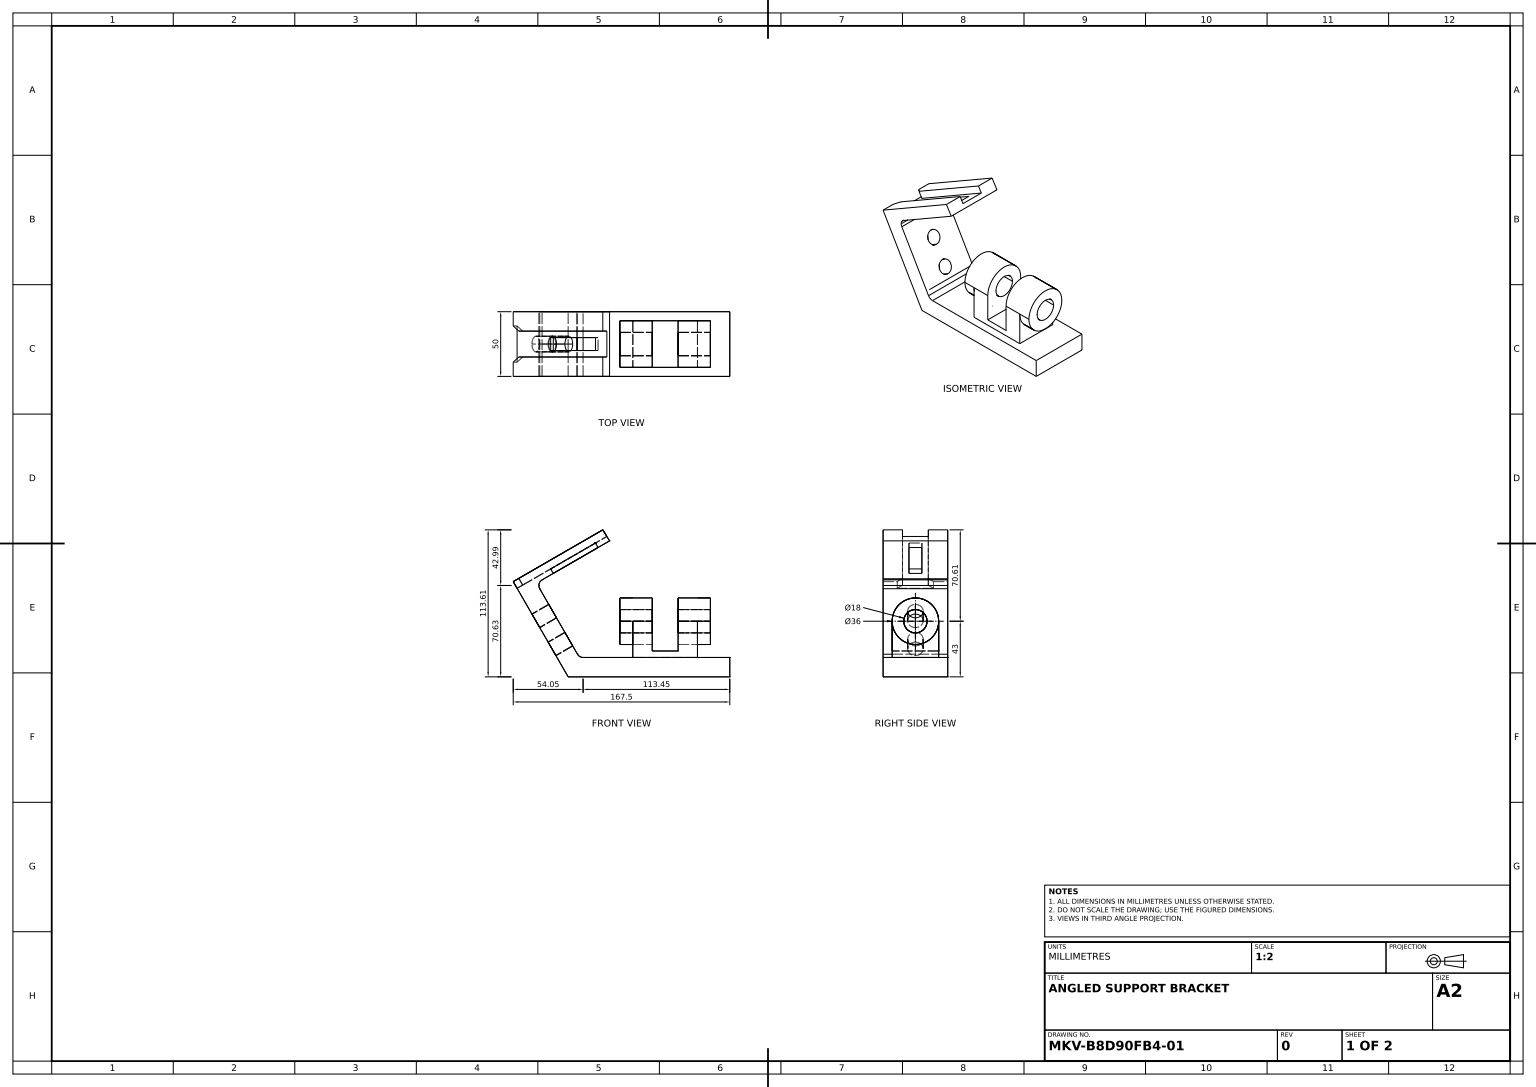
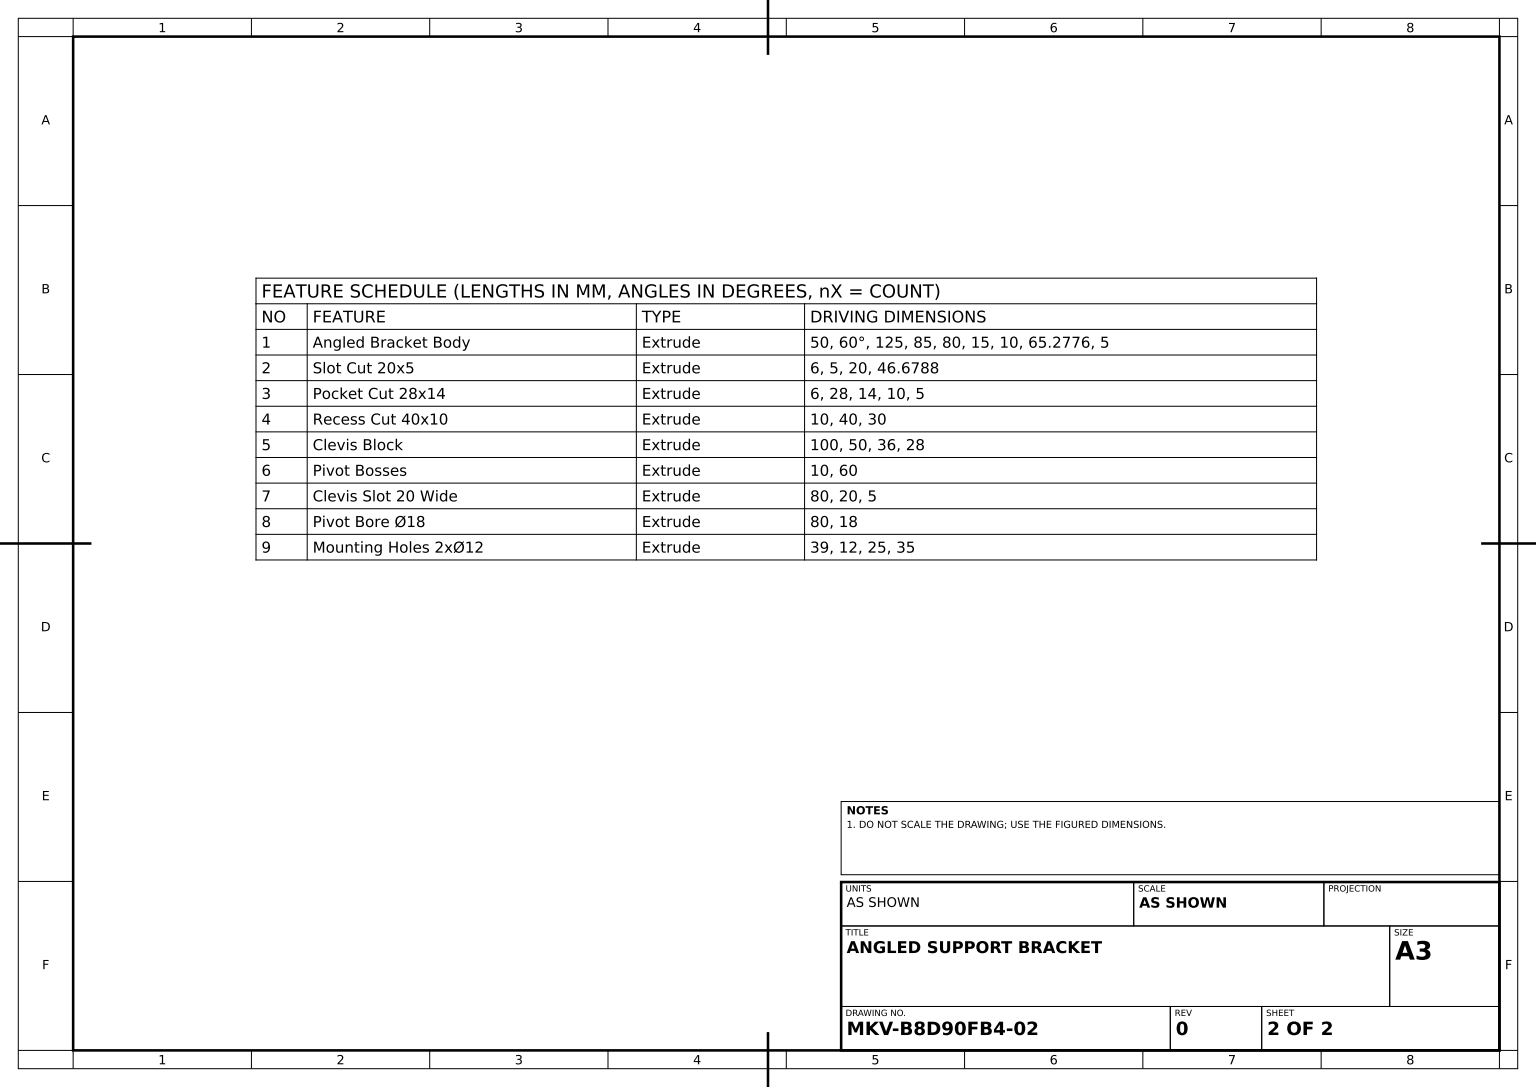
SolidWorks part; units mm, degrees
material "Plain Carbon Steel"
ref_plane "Front Plane" through (0, 0, 0) normal (0, 0, 1) x (1, 0, 0)
ref_plane "Top Plane" through (0, 0, 0) normal (0, 1, 0) x (1, 0, 0)
ref_plane "Right Plane" through (0, 0, 0) normal (1, 0, 0) x (0, 0, -1)
sketch "Bracket Profile Sketch" plane through (0, 0, 0) normal (0, 0, 1) x (1, 0, 0)
  line L0 (0, 103.2476) -> (0, -115.1658) construction
  line L1 (-182.0111, 0) -> (176.8293, 0) construction
  line L2 (125, 0) -> (0, 0)
  line L3 (0, 0) -> (-42.5, 73.6122)
  line L4 (-42.5, 73.6122) -> (26.782, 113.6122)
  line L5 (125, 0) -> (125, 15)
  line L6 (125, 15) -> (11.547, 15)
  line L7 (7.2169, 17.5) -> (-22.0115, 68.1251)
  line L8 (-20.1814, 74.9552) -> (32.0205, 105.0941)
  line L9 (32.0205, 105.0941) -> (26.782, 113.6122)
  arc A0 (-22.0115, 68.1251) -> (-20.1814, 74.9552) centre (-17.6814, 70.6251) cw
  arc A1 (11.547, 15) -> (7.2169, 17.5) centre (11.547, 20) cw
  point P15 (-24.5115, 72.4552)
  dimension "D9" = 5
  dimension "D1" = 60
  dimension "D2" = 125
  dimension "D3" = 85
  dimension "D4" = 80
  dimension "D5" = 15
  dimension "D6" = 15
  dimension "D7" = 10
  dimension "D8" = 65.2776
extrude "Angled Bracket Body" add sketch "Bracket Profile Sketch" along normal mid plane 50
sketch "Slot 20x5 Sketch" plane through (-42.5, 73.6122, 0) normal (-0.5, 0.866, 0) x (0.866, 0.5, 0)
  line L0 (0, -25) -> (0, 25) construction
  line L1 (5, 10) -> (88.3575, 10)
  line L2 (5, 10) -> (5, -10)
  line L3 (5, -10) -> (88.3575, -10)
  line L4 (88.3575, 10) -> (88.3575, -10)
  line L5 (5, 10) -> (88.3575, -10) construction
  line L6 (5, -10) -> (88.3575, 10) construction
  point P0 (46.6788, 0)
  dimension "D1" = 5
  dimension "D2" = 20
  dimension "D3" = 46.6788
extrude "Slot Cut 20x5" cut sketch "Slot 20x5 Sketch" against normal blind 6 contours L3 L4 L1 L2
sketch "Pocket 28x14 Sketch" plane through (-42.5, 73.6122, 0) normal (-0.5, 0.866, 0) x (0.866, 0.5, 0)
  line L0 (0, 14) -> (0, -14)
  line L1 (0, -25) -> (0, 25) construction
  line L2 (5, 10) -> (5, -10)
  line L3 (-13.7994, 0) -> (10.2485, 0) construction
  line L4 (0, 14) -> (5, 10)
  line L5 (5, -10) -> (0, -14)
  dimension "D1" = 28
  dimension "D2" = 14
  dimension "D3" = 10
  dimension "D4" = 10
  dimension "D5" = 5
extrude "Pocket Cut 28x14" cut sketch "Pocket 28x14 Sketch" against normal blind 6
sketch "Recess 40x10 Sketch" plane through (-39.5, 68.416, 0) normal (-0.5, 0.866, 0) x (0.866, 0.5, 0)
  line L1 (30, 5) -> (70, 5)
  line L2 (30, 5) -> (30, -5)
  line L3 (30, -5) -> (70, -5)
  line L4 (70, 5) -> (70, -5)
  line L5 (30, 5) -> (70, -5) construction
  line L6 (30, -5) -> (70, 5) construction
  line L7 (0, 14) -> (0, -14) construction
  point P0 (50, 0)
  dimension "D1" = 30
  dimension "D2" = 40
  dimension "D3" = 10
extrude "Recess Cut 40x10" cut sketch "Recess 40x10 Sketch" against normal blind 10
ref_plane "Clevis Block Plane" through (100, 0, 0) normal (1, 0, 0) x (0, 0, -1)
sketch "Clevis Block Sketch" plane through (100, 0, 0) normal (1, 0, 0) x (0, 0, -1)
  line L0 (-25, 15) -> (25, 15) construction
  line L1 (18, 15) -> (-18, 15)
  line L2 (18, 15) -> (18, 43)
  line L3 (18, 43) -> (-18, 43)
  line L4 (-18, 15) -> (-18, 43)
  line L8 (0, -11.2648) -> (0, 65.9892) construction
  dimension "D1" = 36
  dimension "D2" = 28
extrude "Clevis Block" add sketch "Clevis Block Sketch" against normal blind 50 contours L4 L3 L2 L1
sketch "Pivot Boss Sketch" plane through (100, 0, 0) normal (1, 0, 0) x (0, 0, -1)
  line L0 (18, 43) -> (-18, 43) construction
  circle A0 centre (0, 43) radius 18
extrude "Pivot Bosses" add sketch "Pivot Boss Sketch" along normal blind 10 and the other way blind 60
sketch "Clevis Slot Sketch" plane through (0, 0, 18) normal (0, 0, 1) x (1, 0, 0)
  line L0 (50, 43) -> (100, 43) construction
  line L1 (65, 66) -> (85, 66)
  line L2 (65, 66) -> (65, 20)
  line L3 (65, 20) -> (85, 20)
  line L4 (85, 66) -> (85, 20)
  line L5 (65, 66) -> (85, 20) construction
  line L6 (65, 20) -> (85, 66) construction
  line L7 (50, 15) -> (100, 15) construction
  point P0 (75, 43)
  dimension "D1" = 20
  dimension "D2" = 5
extrude "Clevis Slot 20 Wide" cut sketch "Clevis Slot Sketch" against normal blind 80
sketch "Pivot Bore Sketch" plane through (110, 0, 0) normal (1, 0, 0) x (0, 0, -1)
  circle A0 centre (0, 43) radius 9
  dimension "D1" = 18
extrude "Pivot Bore Ø18" cut sketch "Pivot Bore Sketch" against normal blind 80
sketch "Mounting Holes Sketch" plane through (0, 0, 0) normal (-0.866, -0.5, 0) x (0, 0, 1)
  line L4 (-25, 85) -> (-25, 0) construction
  line L6 (25, 85) -> (14, 85) construction
  circle A0 centre (0, 50) radius 6
  circle A1 centre (0, 25) radius 6
  dimension "D1" = 12
  dimension "D2" = 12
  dimension "D3" = 25
  dimension "D4" = 35
  dimension "D5" = 25
extrude "Mounting Holes 2xØ12" cut sketch "Mounting Holes Sketch" against normal blind 39 contours A0 | A1
